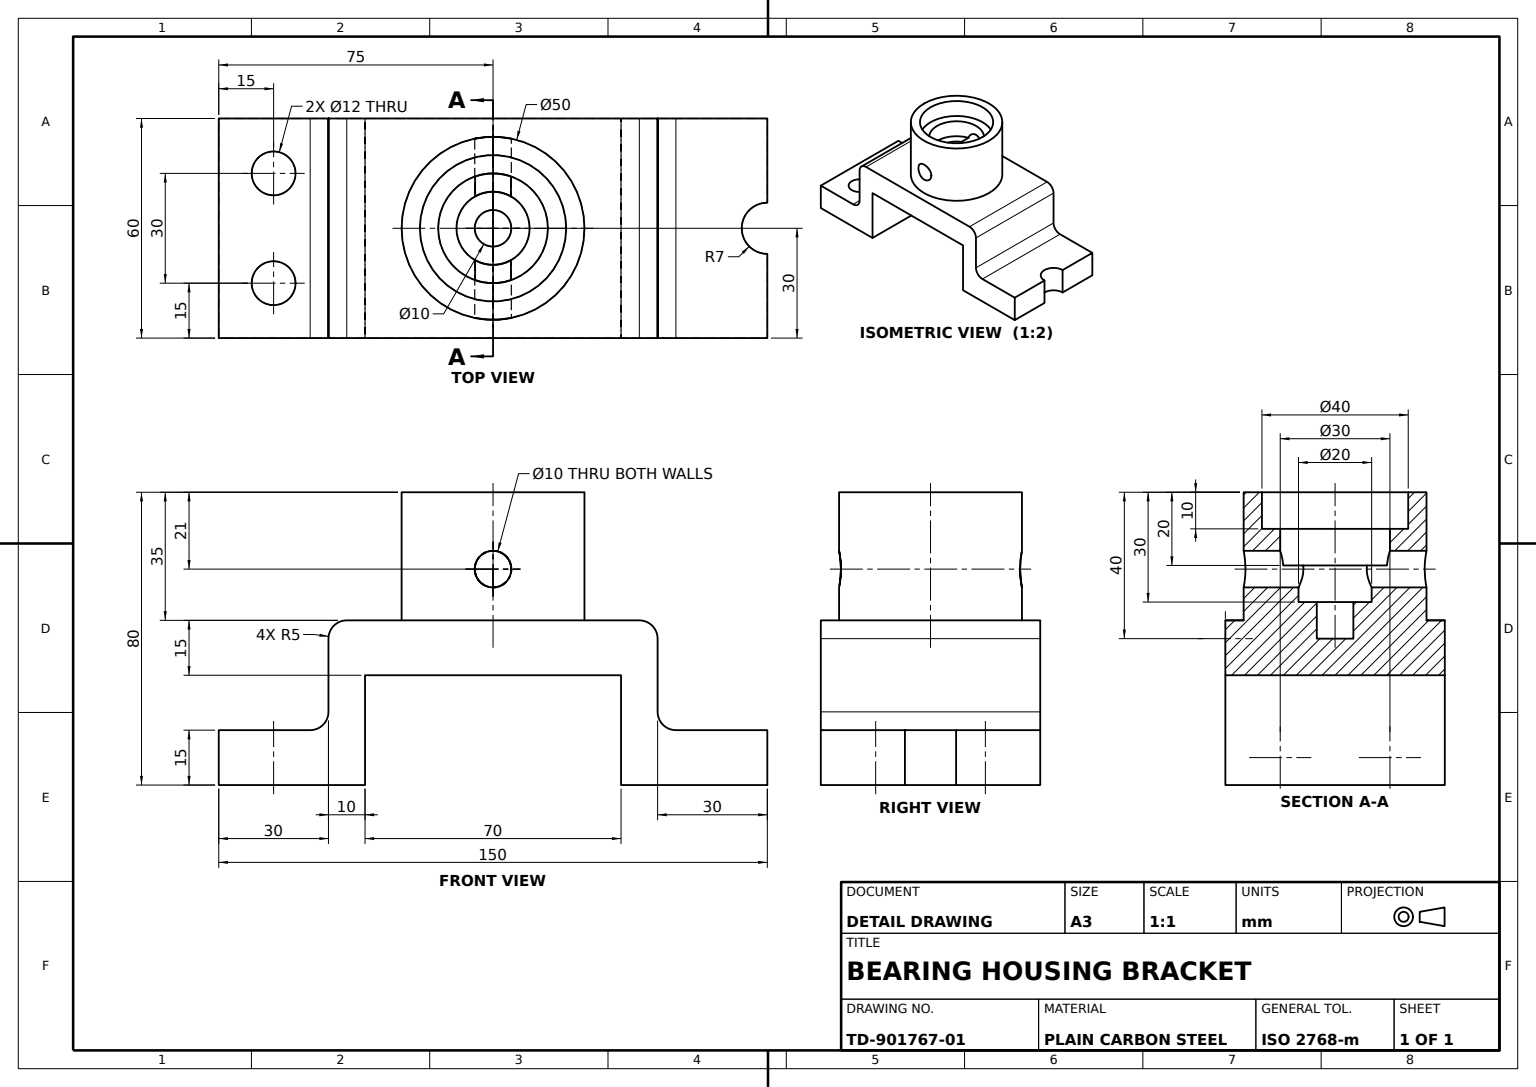
SolidWorks part; units mm, degrees
material "Plain Carbon Steel"
ref_plane "Front Plane" through (0, 0, 0) normal (0, 0, 1) x (1, 0, 0)
ref_plane "Top Plane" through (0, 0, 0) normal (0, 1, 0) x (1, 0, 0)
ref_plane "Right Plane" through (0, 0, 0) normal (1, 0, 0) x (0, 0, -1)
sketch "Bracket Profile Sketch" plane through (0, 0, 0) normal (0, 0, 1) x (1, 0, 0)
  line L0 (-75, -30) -> (-35, -30)
  line L1 (-35, -30) -> (-35, 0)
  line L2 (-35, 0) -> (35, 0)
  line L3 (35, 0) -> (35, -30)
  line L4 (35, -30) -> (75, -30)
  line L5 (75, -30) -> (75, -15)
  line L6 (75, -15) -> (45, -15)
  line L7 (45, -15) -> (45, 15)
  line L8 (45, 15) -> (-45, 15)
  line L9 (-45, 15) -> (-45, -15)
  line L10 (-45, -15) -> (-75, -15)
  line L11 (-75, -30) -> (-75, -15)
  dimension "D1" = 40
  dimension "D2" = 70
  dimension "D3" = 40
  dimension "D4" = 15
  dimension "D5" = 15
  dimension "D6" = 45
  dimension "D7" = 45
  dimension "D9" = 45
  dimension "D10" = 45
extrude "Bracket Body" add sketch "Bracket Profile Sketch" along normal mid plane 60
sketch "Foot Slot A Sketch" plane through (0, -15, 0) normal (0, 1, 0) x (1, 0, 0)
  line L0 (-75, -30) -> (-75, 30) construction
  circle A0 centre (-60, 15) radius 6
  circle A1 centre (-60, -15) radius 6
  dimension "D1" = 12
  dimension "D2" = 15
  dimension "D5" = 15
  dimension "D3" = 15
  dimension "D4" = 30
extrude "Foot Slot A" cut sketch "Foot Slot A Sketch" against normal up to next
sketch "Foot Slot B Sketch" plane through (0, -15, 0) normal (0, 1, 0) x (1, 0, 0)
  line L0 (75, -30) -> (75, 30) construction
  line L1 (75, 7) -> (75, -7)
  arc A0 (75, 7) -> (75, -7) centre (75, 0) ccw
  dimension "D1" = 7
extrude "Foot Slot B" cut sketch "Foot Slot B Sketch" against normal up to next
sketch "Bearing Boss Sketch" plane through (0, 15, 0) normal (0, 1, 0) x (1, 0, 0)
  circle A0 centre (0, 0) radius 25
  dimension "D1" = 50
extrude "Bearing Boss" add sketch "Bearing Boss Sketch" along normal blind 35
sketch "Bore Step 1 Sketch" plane through (0, 50, 0) normal (0, 1, 0) x (1, 0, 0)
  circle A0 centre (0, 0) radius 20
  dimension "D1" = 40
extrude "Bore Step 1" cut sketch "Bore Step 1 Sketch" against normal blind 10
sketch "Bore Step 2 Sketch" plane through (0, 40, 0) normal (0, 1, 0) x (1, 0, 0)
  circle A0 centre (0, 0) radius 15
  dimension "D1" = 30
extrude "Bore Step 2" cut sketch "Bore Step 2 Sketch" against normal blind 10
sketch "Bore Step 3 Sketch" plane through (0, 30, 0) normal (0, 1, 0) x (1, 0, 0)
  circle A0 centre (0, 0) radius 10
  dimension "D1" = 20
extrude "Bore Step 3" cut sketch "Bore Step 3 Sketch" against normal blind 10
sketch "Bore Step 4 Sketch" plane through (0, 20, 0) normal (0, 1, 0) x (1, 0, 0)
  circle A0 centre (0, 0) radius 5
  dimension "D1" = 10
extrude "Bore Step 4" cut sketch "Bore Step 4 Sketch" against normal blind 10
sketch "Cross Hole Sketch" plane through (0, 0, 30) normal (0, 0, 1) x (1, 0, 0)
  line L0 (25, 50) -> (-25, 50) construction
  line L1 (-75, -15) -> (-75, -30) construction
  circle A0 centre (0, 29) radius 5
  dimension "D1" = 21
  dimension "D2" = 10
  dimension "D3" = 75
extrude "Cross Hole" cut sketch "Cross Hole Sketch" against normal through all
fillet "Bend Fillet R5 A" radius 5 1 edges at (45, -15, 0)
fillet "Bend Fillet R5 B" radius 5 2 edges at (-45, 15, 0) (45, 15, 0)
fillet "Bend Fillet R5 C" radius 5 1 edges at (-45, -15, 0)
